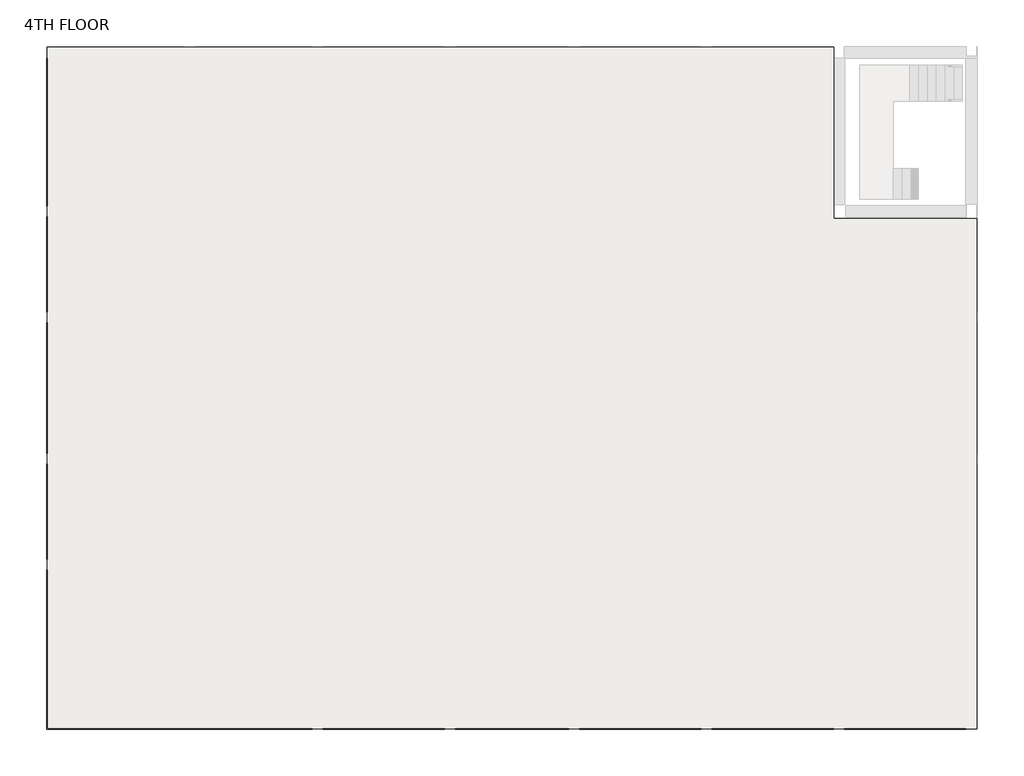
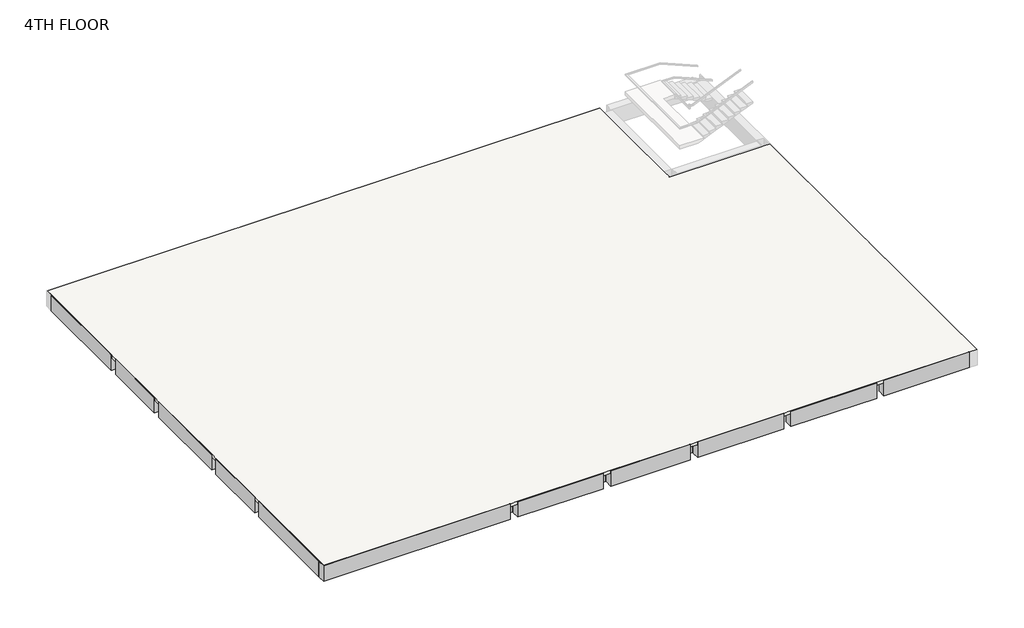
# One storey, part 1 of 2: 9 beams, 1 slab.
"""IFC4 building model written with IfcOpenShell, lengths in millimetres."""

from ifc_helpers import new_model, si_unit, frame, origin, place, context, project, spatial, polyline, outline, extrude, faceted_brep, element, save

model = new_model("IFC4")

# Units and contexts
model_context = context("Model", 3, world=origin())
ifc_project = project(units=[si_unit("LENGTHUNIT", "METRE", prefix="MILLI")], contexts=[model_context])

# Site, building, storey
site = spatial("IfcSite", under=ifc_project)
building = spatial("IfcBuilding", under=site)
storey = spatial("IfcBuildingStorey", under=building, Name="4TH FLOOR", Elevation=13716.0)

# Beams
placement = place(None, origin())
element("IfcBeam", 1, ObjectType="M_Concrete-Rectangular Beam : 400 x 800mm", at=placement, inside=storey, context=model_context, shape_type="Brep", body=[
    faceted_brep([(-25701.5491019, -6047.8309165, 13716.0), (-25701.5491019, -6447.8309165, 13716.0), (-16535.3491019, -6447.8309165, 13716.0), (-16535.3491019, -6425.6309165, 13716.0), (-25679.3491019, -6425.6309165, 13716.0), (-25679.3491019, -6047.8309165, 13716.0), (-25701.5491019, -6047.8309165, 12916.0), (-25679.3491019, -6047.8309165, 13563.6), (-25301.5491019, -6047.8309165, 13563.6), (-20977.1491019, -6047.8309165, 13563.6), (-20577.1491019, -6047.8309165, 13563.6), (-16557.5491019, -6047.8309165, 13563.6), (-16535.3491019, -6047.8309165, 13563.6), (-16535.3491019, -6047.8309165, 12916.0), (-16557.5491019, -6047.8309165, 12916.0), (-20577.1491019, -6047.8309165, 12916.0), (-20977.1491019, -6047.8309165, 12916.0), (-25301.5491019, -6047.8309165, 12916.0), (-25701.5491019, -6447.8309165, 12916.0), (-16535.3491019, -6447.8309165, 12916.0), (-25323.7491019, -6425.6309165, 12916.0), (-25323.7491019, -6070.0309165, 12916.0), (-25679.3491019, -6070.0309165, 12916.0), (-25679.3491019, -6425.6309165, 12916.0), (-20599.3491019, -6425.6309165, 12916.0), (-20599.3491019, -6070.0309165, 12916.0), (-20954.9491019, -6070.0309165, 12916.0), (-20954.9491019, -6425.6309165, 12916.0), (-25323.7491019, -6425.6309165, 13563.6), (-25323.7491019, -6070.0309165, 13563.6), (-16535.3491019, -6425.6309165, 13563.6), (-20599.3491019, -6425.6309165, 13563.6), (-20954.9491019, -6425.6309165, 13563.6), (-25679.3491019, -6425.6309165, 13563.6), (-25679.3491019, -6070.0309165, 13563.6), (-20599.3491019, -6070.0309165, 13563.6), (-20954.9491019, -6070.0309165, 13563.6)], [[[0, 1, 2, 3, 4, 5]], [[6, 0, 5, 7, 8, 9, 10, 11, 12, 13, 14, 15, 16, 17]], [[18, 6, 17, 16, 15, 14, 13, 19], [20, 21, 22, 23], [24, 25, 26, 27]], [[1, 18, 19, 2]], [[1, 0, 6, 18]], [[21, 20, 28, 29]], [[30, 31, 24, 27, 32, 28, 20, 23, 33, 4, 3]], [[4, 33, 23, 22, 34, 7, 5]], [[22, 21, 29, 34]], [[25, 24, 31, 35]], [[27, 26, 36, 32]], [[26, 25, 35, 36]], [[19, 13, 12, 30, 3, 2]], [[28, 32, 36, 35, 31, 30, 12, 11, 10, 9, 8, 7, 34, 29]]]),
    faceted_brep([(5997.6508981, -6447.8309165, 12916.0), (5997.6508981, -6047.8309165, 12916.0), (5997.6508981, -6047.8309165, 13563.6), (5997.6508981, -6425.6309165, 13563.6), (5997.6508981, -6425.6309165, 13716.0), (5997.6508981, -6447.8309165, 13716.0), (1803.4508981, -6047.8309165, 12916.0), (1803.4508981, -6447.8309165, 12916.0), (1803.4508981, -6447.8309165, 13716.0), (1803.4508981, -6425.6309165, 13716.0), (1803.4508981, -6425.6309165, 13563.6), (1803.4508981, -6047.8309165, 13563.6), (1825.6508981, -6047.8309165, 12916.0), (1825.6508981, -6047.8309165, 13563.6)], [[[0, 1, 2, 3, 4, 5]], [[6, 7, 8, 9, 10, 11]], [[8, 5, 4, 9]], [[1, 12, 6, 11, 13, 2]], [[1, 0, 7, 6, 12]], [[0, 5, 8, 7]], [[10, 3, 2, 13, 11]], [[3, 10, 9, 4]]]),
    faceted_brep([(-16179.7491019, -6047.8309165, 12916.0), (-16179.7491019, -6447.8309165, 12916.0), (-16179.7491019, -6447.8309165, 13716.0), (-16179.7491019, -6425.6309165, 13716.0), (-16179.7491019, -6425.6309165, 13563.6), (-16179.7491019, -6047.8309165, 13563.6), (-11963.3491019, -6447.8309165, 13716.0), (-11963.3491019, -6425.6309165, 13716.0), (-11963.3491019, -6047.8309165, 12916.0), (-11985.5491019, -6047.8309165, 12916.0), (-16157.5491019, -6047.8309165, 12916.0), (-16157.5491019, -6047.8309165, 13563.6), (-11985.5491019, -6047.8309165, 13563.6), (-11963.3491019, -6047.8309165, 13563.6), (-11963.3491019, -6447.8309165, 12916.0), (-11963.3491019, -6425.6309165, 13563.6)], [[[0, 1, 2, 3, 4, 5]], [[2, 6, 7, 3]], [[8, 9, 10, 0, 5, 11, 12, 13]], [[1, 0, 10, 9, 8, 14]], [[2, 1, 14, 6]], [[14, 8, 13, 15, 7, 6]], [[15, 4, 3, 7]], [[4, 15, 13, 12, 11, 5]]]),
    faceted_brep([(-11607.7491019, -6047.8309165, 12916.0), (-11607.7491019, -6447.8309165, 12916.0), (-11607.7491019, -6447.8309165, 13716.0), (-11607.7491019, -6425.6309165, 13716.0), (-11607.7491019, -6425.6309165, 13563.6), (-11607.7491019, -6047.8309165, 13563.6), (-7696.1491019, -6447.8309165, 13716.0), (-7696.1491019, -6425.6309165, 13716.0), (-7696.1491019, -6047.8309165, 12916.0), (-7718.3491019, -6047.8309165, 12916.0), (-11585.5491019, -6047.8309165, 12916.0), (-11585.5491019, -6047.8309165, 13563.6), (-7718.3491019, -6047.8309165, 13563.6), (-7696.1491019, -6047.8309165, 13563.6), (-7696.1491019, -6447.8309165, 12916.0), (-7696.1491019, -6425.6309165, 13563.6)], [[[0, 1, 2, 3, 4, 5]], [[2, 6, 7, 3]], [[8, 9, 10, 0, 5, 11, 12, 13]], [[1, 0, 10, 9, 8, 14]], [[2, 1, 14, 6]], [[14, 8, 13, 15, 7, 6]], [[15, 4, 3, 7]], [[4, 15, 13, 12, 11, 5]]]),
    faceted_brep([(-7340.5491019, -6047.8309165, 12916.0), (-7340.5491019, -6447.8309165, 12916.0), (-7340.5491019, -6447.8309165, 13716.0), (-7340.5491019, -6425.6309165, 13716.0), (-7340.5491019, -6425.6309165, 13563.6), (-7340.5491019, -6047.8309165, 13563.6), (-3124.1491019, -6447.8309165, 13716.0), (-3124.1491019, -6425.6309165, 13716.0), (-3124.1491019, -6047.8309165, 12916.0), (-3146.3491019, -6047.8309165, 12916.0), (-7318.3491019, -6047.8309165, 12916.0), (-7318.3491019, -6047.8309165, 13563.6), (-3146.3491019, -6047.8309165, 13563.6), (-3124.1491019, -6047.8309165, 13563.6), (-3124.1491019, -6447.8309165, 12916.0), (-3124.1491019, -6425.6309165, 13563.6)], [[[0, 1, 2, 3, 4, 5]], [[2, 6, 7, 3]], [[8, 9, 10, 0, 5, 11, 12, 13]], [[1, 0, 10, 9, 8, 14]], [[2, 1, 14, 6]], [[14, 8, 13, 15, 7, 6]], [[15, 4, 3, 7]], [[4, 15, 13, 12, 11, 5]]]),
    faceted_brep([(-2768.5491019, -6047.8309165, 12916.0), (-2768.5491019, -6447.8309165, 12916.0), (-2768.5491019, -6447.8309165, 13716.0), (-2768.5491019, -6425.6309165, 13716.0), (-2768.5491019, -6425.6309165, 13563.6), (-2768.5491019, -6047.8309165, 13563.6), (1447.8508981, -6447.8309165, 13716.0), (1447.8508981, -6425.6309165, 13716.0), (1447.8508981, -6047.8309165, 12916.0), (1425.6508981, -6047.8309165, 12916.0), (-2746.3491019, -6047.8309165, 12916.0), (-2746.3491019, -6047.8309165, 13563.6), (1425.6508981, -6047.8309165, 13563.6), (1447.8508981, -6047.8309165, 13563.6), (1447.8508981, -6447.8309165, 12916.0), (1447.8508981, -6425.6309165, 13563.6)], [[[0, 1, 2, 3, 4, 5]], [[2, 6, 7, 3]], [[8, 9, 10, 0, 5, 11, 12, 13]], [[1, 0, 10, 9, 8, 14]], [[2, 1, 14, 6]], [[14, 8, 13, 15, 7, 6]], [[15, 4, 3, 7]], [[4, 15, 13, 12, 11, 5]]]),
])
element("IfcBeam", 2, ObjectType="M_Concrete-Rectangular Beam : 400 x 800mm", at=placement, inside=storey, context=model_context, shape_type="Brep", body=[
    faceted_brep([(-25701.5491019, -939.2309165, 13716.0), (-25701.5491019, -6047.8309165, 13716.0), (-25679.3491019, -6047.8309165, 13716.0), (-25679.3491019, -939.2309165, 13716.0), (-25301.5491019, -6047.8309165, 12916.0), (-25301.5491019, -961.4309165, 12916.0), (-25301.5491019, -939.2309165, 12916.0), (-25301.5491019, -939.2309165, 13563.6), (-25301.5491019, -961.4309165, 13563.6), (-25301.5491019, -6047.8309165, 13563.6), (-25701.5491019, -6047.8309165, 12916.0), (-25701.5491019, -939.2309165, 12916.0), (-25679.3491019, -6047.8309165, 13563.6), (-25679.3491019, -939.2309165, 13563.6)], [[[0, 1, 2, 3]], [[4, 5, 6, 7, 8, 9]], [[4, 10, 11, 6, 5]], [[10, 1, 0, 11]], [[10, 4, 9, 12, 2, 1]], [[6, 11, 0, 3, 13, 7]], [[12, 13, 3, 2]], [[13, 12, 9, 8, 7]]]),
    faceted_brep([(-25301.5491019, 16716.9690835, 12916.0), (-25701.5491019, 16716.9690835, 12916.0), (-25701.5491019, 16716.9690835, 13716.0), (-25679.3491019, 16716.9690835, 13716.0), (-25679.3491019, 16716.9690835, 13563.6), (-25301.5491019, 16716.9690835, 13563.6), (-25701.5491019, 11608.3690835, 13716.0), (-25679.3491019, 11608.3690835, 13716.0), (-25301.5491019, 11608.3690835, 12916.0), (-25301.5491019, 11630.5690835, 12916.0), (-25301.5491019, 11630.5690835, 13563.6), (-25301.5491019, 11608.3690835, 13563.6), (-25701.5491019, 11608.3690835, 12916.0), (-25679.3491019, 11608.3690835, 13563.6)], [[[0, 1, 2, 3, 4, 5]], [[2, 6, 7, 3]], [[8, 9, 0, 5, 10, 11]], [[1, 0, 9, 8, 12]], [[2, 1, 12, 6]], [[12, 8, 11, 13, 7, 6]], [[4, 13, 11, 10, 5]], [[13, 4, 3, 7]]]),
    faceted_brep([(-25701.5491019, 7950.7690835, 12916.0), (-25301.5491019, 7950.7690835, 12916.0), (-25301.5491019, 7950.7690835, 13563.6), (-25679.3491019, 7950.7690835, 13563.6), (-25679.3491019, 7950.7690835, 13716.0), (-25701.5491019, 7950.7690835, 13716.0), (-25301.5491019, 11252.7690835, 12916.0), (-25701.5491019, 11252.7690835, 12916.0), (-25701.5491019, 11252.7690835, 13716.0), (-25679.3491019, 11252.7690835, 13716.0), (-25679.3491019, 11252.7690835, 13563.6), (-25301.5491019, 11252.7690835, 13563.6), (-25301.5491019, 7972.9690835, 13563.6), (-25301.5491019, 11230.5690835, 13563.6), (-25301.5491019, 7972.9690835, 12916.0), (-25301.5491019, 11230.5690835, 12916.0)], [[[0, 1, 2, 3, 4, 5]], [[6, 7, 8, 9, 10, 11]], [[10, 3, 2, 12, 13, 11]], [[3, 10, 9, 4]], [[8, 5, 4, 9]], [[1, 14, 15, 6, 11, 13, 12, 2]], [[1, 0, 7, 6, 15, 14]], [[0, 5, 8, 7]]]),
    faceted_brep([(-25301.5491019, 7595.1690835, 12916.0), (-25701.5491019, 7595.1690835, 12916.0), (-25701.5491019, 7595.1690835, 13716.0), (-25679.3491019, 7595.1690835, 13716.0), (-25679.3491019, 7595.1690835, 13563.6), (-25301.5491019, 7595.1690835, 13563.6), (-25701.5491019, 3073.9690835, 12916.0), (-25301.5491019, 3073.9690835, 12916.0), (-25301.5491019, 3073.9690835, 13563.6), (-25679.3491019, 3073.9690835, 13563.6), (-25679.3491019, 3073.9690835, 13716.0), (-25701.5491019, 3073.9690835, 13716.0), (-25301.5491019, 3096.1690835, 13563.6), (-25301.5491019, 7572.9690835, 13563.6), (-25301.5491019, 3096.1690835, 12916.0), (-25301.5491019, 7572.9690835, 12916.0)], [[[0, 1, 2, 3, 4, 5]], [[6, 7, 8, 9, 10, 11]], [[4, 9, 8, 12, 13, 5]], [[9, 4, 3, 10]], [[2, 11, 10, 3]], [[7, 14, 15, 0, 5, 13, 12, 8]], [[1, 0, 15, 14, 7, 6]], [[2, 1, 6, 11]]]),
    faceted_brep([(-25301.5491019, 2718.3690835, 12916.0), (-25701.5491019, 2718.3690835, 12916.0), (-25701.5491019, 2718.3690835, 13716.0), (-25679.3491019, 2718.3690835, 13716.0), (-25679.3491019, 2718.3690835, 13563.6), (-25301.5491019, 2718.3690835, 13563.6), (-25701.5491019, -583.6309165, 12916.0), (-25301.5491019, -583.6309165, 12916.0), (-25301.5491019, -583.6309165, 13563.6), (-25679.3491019, -583.6309165, 13563.6), (-25679.3491019, -583.6309165, 13716.0), (-25701.5491019, -583.6309165, 13716.0), (-25301.5491019, -561.4309165, 13563.6), (-25301.5491019, 2696.1690835, 13563.6), (-25301.5491019, -561.4309165, 12916.0), (-25301.5491019, 2696.1690835, 12916.0)], [[[0, 1, 2, 3, 4, 5]], [[6, 7, 8, 9, 10, 11]], [[4, 9, 8, 12, 13, 5]], [[9, 4, 3, 10]], [[2, 11, 10, 3]], [[7, 14, 15, 0, 5, 13, 12, 8]], [[0, 15, 14, 7, 6, 1]], [[11, 2, 1, 6]]]),
])
element("IfcBeam", 3, ObjectType="M_Concrete-Rectangular Beam : 400 x 800mm", at=placement, inside=storey, context=model_context, shape_type="SweptSolid", body=[
    extrude(outline(polyline([(-20577.1491019, -6047.8309165), (-20977.1491019, -6047.8309165), (-20977.1491019, -990.0309165), (-20577.1491019, -990.0309165), (-20577.1491019, -6047.8309165)])), frame((0.0, 0.0, 12916.0), z_axis=(0.0, 0.0, 1.0), x_axis=(1.0, 0.0, 0.0)), (0.0, 0.0, 1.0), 647.6),
    extrude(outline(polyline([(-20599.3491019, 16716.9690835), (-20577.1491019, 16716.9690835), (-20577.1491019, 11659.1690835), (-20977.1491019, 11659.1690835), (-20977.1491019, 16716.9690835), (-20954.9491019, 16716.9690835), (-20954.9491019, 16662.9690835), (-20599.3491019, 16662.9690835), (-20599.3491019, 16716.9690835)])), frame((0.0, 0.0, 12916.0), z_axis=(0.0, 0.0, 1.0), x_axis=(1.0, 0.0, 0.0)), (0.0, 0.0, 1.0), 647.6),
    extrude(outline(polyline([(-20977.1491019, 11201.9690835), (-20577.1491019, 11201.9690835), (-20577.1491019, 8001.5690835), (-20977.1491019, 8001.5690835), (-20977.1491019, 11201.9690835)])), frame((0.0, 0.0, 12916.0), z_axis=(0.0, 0.0, 1.0), x_axis=(1.0, 0.0, 0.0)), (0.0, 0.0, 1.0), 647.6),
    extrude(outline(polyline([(-20977.1491019, 7544.3690835), (-20577.1491019, 7544.3690835), (-20577.1491019, 3124.7690835), (-20977.1491019, 3124.7690835), (-20977.1491019, 7544.3690835)])), frame((0.0, 0.0, 12916.0), z_axis=(0.0, 0.0, 1.0), x_axis=(1.0, 0.0, 0.0)), (0.0, 0.0, 1.0), 647.6),
    extrude(outline(polyline([(-20977.1491019, 2667.5690835), (-20577.1491019, 2667.5690835), (-20577.1491019, -532.8309165), (-20977.1491019, -532.8309165), (-20977.1491019, 2667.5690835)])), frame((0.0, 0.0, 12916.0), z_axis=(0.0, 0.0, 1.0), x_axis=(1.0, 0.0, 0.0)), (0.0, 0.0, 1.0), 647.6),
])
element("IfcBeam", 4, ObjectType="M_Concrete-Rectangular Beam : 400 x 800mm", at=placement, inside=storey, context=model_context, shape_type="SweptSolid", body=[
    extrude(outline(polyline([(-16157.5491019, -6047.8309165), (-16179.7491019, -6047.8309165), (-16179.7491019, -6019.2309165), (-16535.3491019, -6019.2309165), (-16535.3491019, -6047.8309165), (-16557.5491019, -6047.8309165), (-16557.5491019, -990.0309165), (-16157.5491019, -990.0309165), (-16157.5491019, -6047.8309165)])), frame((0.0, 0.0, 12916.0), z_axis=(0.0, 0.0, 1.0), x_axis=(1.0, 0.0, 0.0)), (0.0, 0.0, 1.0), 647.6),
    extrude(outline(polyline([(-16179.7491019, 16716.9690835), (-16157.5491019, 16716.9690835), (-16157.5491019, 11659.1690835), (-16557.5491019, 11659.1690835), (-16557.5491019, 16716.9690835), (-16535.3491019, 16716.9690835), (-16535.3491019, 16688.3690835), (-16179.7491019, 16688.3690835), (-16179.7491019, 16716.9690835)])), frame((0.0, 0.0, 12916.0), z_axis=(0.0, 0.0, 1.0), x_axis=(1.0, 0.0, 0.0)), (0.0, 0.0, 1.0), 647.6),
    extrude(outline(polyline([(-16557.5491019, 11201.9690835), (-16157.5491019, 11201.9690835), (-16157.5491019, 8001.5690835), (-16557.5491019, 8001.5690835), (-16557.5491019, 11201.9690835)])), frame((0.0, 0.0, 12916.0), z_axis=(0.0, 0.0, 1.0), x_axis=(1.0, 0.0, 0.0)), (0.0, 0.0, 1.0), 647.6),
    extrude(outline(polyline([(-16557.5491019, 7544.3690835), (-16157.5491019, 7544.3690835), (-16157.5491019, 3124.7690835), (-16557.5491019, 3124.7690835), (-16557.5491019, 7544.3690835)])), frame((0.0, 0.0, 12916.0), z_axis=(0.0, 0.0, 1.0), x_axis=(1.0, 0.0, 0.0)), (0.0, 0.0, 1.0), 647.6),
    extrude(outline(polyline([(-16557.5491019, 2667.5690835), (-16157.5491019, 2667.5690835), (-16157.5491019, -532.8309165), (-16557.5491019, -532.8309165), (-16557.5491019, 2667.5690835)])), frame((0.0, 0.0, 12916.0), z_axis=(0.0, 0.0, 1.0), x_axis=(1.0, 0.0, 0.0)), (0.0, 0.0, 1.0), 647.6),
])
element("IfcBeam", 5, ObjectType="M_Concrete-Rectangular Beam : 400 x 800mm", at=placement, inside=storey, context=model_context, shape_type="SweptSolid", body=[
    extrude(outline(polyline([(-11585.5491019, -6047.8309165), (-11607.7491019, -6047.8309165), (-11607.7491019, -6019.2309165), (-11963.3491019, -6019.2309165), (-11963.3491019, -6047.8309165), (-11985.5491019, -6047.8309165), (-11985.5491019, -990.0309165), (-11585.5491019, -990.0309165), (-11585.5491019, -6047.8309165)])), frame((0.0, 0.0, 12916.0), z_axis=(0.0, 0.0, 1.0), x_axis=(1.0, 0.0, 0.0)), (0.0, 0.0, 1.0), 647.6),
    extrude(outline(polyline([(-11607.7491019, 16716.9690835), (-11585.5491019, 16716.9690835), (-11585.5491019, 11659.1690835), (-11985.5491019, 11659.1690835), (-11985.5491019, 16716.9690835), (-11963.3491019, 16716.9690835), (-11963.3491019, 16688.3690835), (-11607.7491019, 16688.3690835), (-11607.7491019, 16716.9690835)])), frame((0.0, 0.0, 12916.0), z_axis=(0.0, 0.0, 1.0), x_axis=(1.0, 0.0, 0.0)), (0.0, 0.0, 1.0), 647.6),
    extrude(outline(polyline([(-11985.5491019, 11201.9690835), (-11585.5491019, 11201.9690835), (-11585.5491019, 8001.5690835), (-11985.5491019, 8001.5690835), (-11985.5491019, 11201.9690835)])), frame((0.0, 0.0, 12916.0), z_axis=(0.0, 0.0, 1.0), x_axis=(1.0, 0.0, 0.0)), (0.0, 0.0, 1.0), 647.6),
    extrude(outline(polyline([(-11985.5491019, 7544.3690835), (-11585.5491019, 7544.3690835), (-11585.5491019, 3124.7690835), (-11985.5491019, 3124.7690835), (-11985.5491019, 7544.3690835)])), frame((0.0, 0.0, 12916.0), z_axis=(0.0, 0.0, 1.0), x_axis=(1.0, 0.0, 0.0)), (0.0, 0.0, 1.0), 647.6),
    extrude(outline(polyline([(-11585.5491019, -532.8309165), (-11985.5491019, -532.8309165), (-11985.5491019, 2667.5690835), (-11585.5491019, 2667.5690835), (-11585.5491019, -532.8309165)])), frame((0.0, 0.0, 12916.0), z_axis=(0.0, 0.0, 1.0), x_axis=(1.0, 0.0, 0.0)), (0.0, 0.0, 1.0), 647.6),
])
element("IfcBeam", 6, ObjectType="M_Concrete-Rectangular Beam : 400 x 800mm", at=placement, inside=storey, context=model_context, shape_type="SweptSolid", body=[
    extrude(outline(polyline([(-7318.3491019, -6047.8309165), (-7340.5491019, -6047.8309165), (-7340.5491019, -6019.2309165), (-7696.1491019, -6019.2309165), (-7696.1491019, -6047.8309165), (-7718.3491019, -6047.8309165), (-7718.3491019, -990.0309165), (-7318.3491019, -990.0309165), (-7318.3491019, -6047.8309165)])), frame((0.0, 0.0, 12916.0), z_axis=(0.0, 0.0, 1.0), x_axis=(1.0, 0.0, 0.0)), (0.0, 0.0, 1.0), 647.6),
    extrude(outline(polyline([(-7340.5491019, 16716.9690835), (-7318.3491019, 16716.9690835), (-7318.3491019, 11659.1690835), (-7718.3491019, 11659.1690835), (-7718.3491019, 16716.9690835), (-7696.1491019, 16716.9690835), (-7696.1491019, 16688.3690835), (-7340.5491019, 16688.3690835), (-7340.5491019, 16716.9690835)])), frame((0.0, 0.0, 12916.0), z_axis=(0.0, 0.0, 1.0), x_axis=(1.0, 0.0, 0.0)), (0.0, 0.0, 1.0), 647.6),
    extrude(outline(polyline([(-7718.3491019, 7544.3690835), (-7318.3491019, 7544.3690835), (-7318.3491019, 3124.7690835), (-7718.3491019, 3124.7690835), (-7718.3491019, 7544.3690835)])), frame((0.0, 0.0, 12916.0), z_axis=(0.0, 0.0, 1.0), x_axis=(1.0, 0.0, 0.0)), (0.0, 0.0, 1.0), 647.6),
    extrude(outline(polyline([(-7318.3491019, 8001.5690835), (-7718.3491019, 8001.5690835), (-7718.3491019, 11201.9690835), (-7318.3491019, 11201.9690835), (-7318.3491019, 8001.5690835)])), frame((0.0, 0.0, 12916.0), z_axis=(0.0, 0.0, 1.0), x_axis=(1.0, 0.0, 0.0)), (0.0, 0.0, 1.0), 647.6),
    extrude(outline(polyline([(-7318.3491019, -532.8309165), (-7718.3491019, -532.8309165), (-7718.3491019, 2667.5690835), (-7318.3491019, 2667.5690835), (-7318.3491019, -532.8309165)])), frame((0.0, 0.0, 12916.0), z_axis=(0.0, 0.0, 1.0), x_axis=(1.0, 0.0, 0.0)), (0.0, 0.0, 1.0), 647.6),
])
element("IfcBeam", 7, ObjectType="M_Concrete-Rectangular Beam : 400 x 800mm", at=placement, inside=storey, context=model_context, shape_type="SweptSolid", body=[
    extrude(outline(polyline([(-25301.5491019, 3073.9690835), (-25301.5491019, 3096.1690835), (-21005.7491019, 3096.1690835), (-21005.7491019, 2696.1690835), (-25301.5491019, 2696.1690835), (-25301.5491019, 2718.3690835), (-25272.9491019, 2718.3690835), (-25272.9491019, 3073.9690835), (-25301.5491019, 3073.9690835)])), frame((0.0, 0.0, 12916.0), z_axis=(0.0, 0.0, 1.0), x_axis=(1.0, 0.0, 0.0)), (0.0, 0.0, 1.0), 647.6),
    extrude(outline(polyline([(5997.6508981, 3096.1690835), (5997.6508981, 3073.9690835), (5969.0508981, 3073.9690835), (5969.0508981, 2718.3690835), (5997.6508981, 2718.3690835), (5997.6508981, 2696.1690835), (1854.2508981, 2696.1690835), (1854.2508981, 3096.1690835), (5997.6508981, 3096.1690835)])), frame((0.0, 0.0, 12916.0), z_axis=(0.0, 0.0, 1.0), x_axis=(1.0, 0.0, 0.0)), (0.0, 0.0, 1.0), 647.6),
    extrude(outline(polyline([(-20548.5491019, 2696.1690835), (-20548.5491019, 3096.1690835), (-16586.1491019, 3096.1690835), (-16586.1491019, 2696.1690835), (-20548.5491019, 2696.1690835)])), frame((0.0, 0.0, 12916.0), z_axis=(0.0, 0.0, 1.0), x_axis=(1.0, 0.0, 0.0)), (0.0, 0.0, 1.0), 647.6),
    extrude(outline(polyline([(-16128.9491019, 2696.1690835), (-16128.9491019, 3096.1690835), (-12014.1491019, 3096.1690835), (-12014.1491019, 2696.1690835), (-16128.9491019, 2696.1690835)])), frame((0.0, 0.0, 12916.0), z_axis=(0.0, 0.0, 1.0), x_axis=(1.0, 0.0, 0.0)), (0.0, 0.0, 1.0), 647.6),
    extrude(outline(polyline([(1397.0508981, 3096.1690835), (1397.0508981, 2696.1690835), (-2717.7491019, 2696.1690835), (-2717.7491019, 3096.1690835), (1397.0508981, 3096.1690835)])), frame((0.0, 0.0, 12916.0), z_axis=(0.0, 0.0, 1.0), x_axis=(1.0, 0.0, 0.0)), (0.0, 0.0, 1.0), 647.6),
    extrude(outline(polyline([(-3174.9491019, 3096.1690835), (-3174.9491019, 2696.1690835), (-7289.7491019, 2696.1690835), (-7289.7491019, 3096.1690835), (-3174.9491019, 3096.1690835)])), frame((0.0, 0.0, 12916.0), z_axis=(0.0, 0.0, 1.0), x_axis=(1.0, 0.0, 0.0)), (0.0, 0.0, 1.0), 647.6),
    extrude(outline(polyline([(-7746.9491019, 3096.1690835), (-7746.9491019, 2696.1690835), (-11556.9491019, 2696.1690835), (-11556.9491019, 3096.1690835), (-7746.9491019, 3096.1690835)])), frame((0.0, 0.0, 12916.0), z_axis=(0.0, 0.0, 1.0), x_axis=(1.0, 0.0, 0.0)), (0.0, 0.0, 1.0), 647.6),
])
element("IfcBeam", 8, ObjectType="M_Concrete-Rectangular Beam : 400 x 800mm", at=placement, inside=storey, context=model_context, shape_type="SweptSolid", body=[
    extrude(outline(polyline([(-25301.5491019, -583.6309165), (-25301.5491019, -561.4309165), (-21005.7491019, -561.4309165), (-21005.7491019, -961.4309165), (-25301.5491019, -961.4309165), (-25301.5491019, -939.2309165), (-25247.5491019, -939.2309165), (-25247.5491019, -583.6309165), (-25301.5491019, -583.6309165)])), frame((0.0, 0.0, 12916.0), z_axis=(0.0, 0.0, 1.0), x_axis=(1.0, 0.0, 0.0)), (0.0, 0.0, 1.0), 647.6),
    extrude(outline(polyline([(5997.6508981, -561.4309165), (5997.6508981, -961.4309165), (1854.2508981, -961.4309165), (1854.2508981, -561.4309165), (5997.6508981, -561.4309165)])), frame((0.0, 0.0, 12916.0), z_axis=(0.0, 0.0, 1.0), x_axis=(1.0, 0.0, 0.0)), (0.0, 0.0, 1.0), 647.6),
    extrude(outline(polyline([(-20548.5491019, -961.4309165), (-20548.5491019, -561.4309165), (-16586.1491019, -561.4309165), (-16586.1491019, -961.4309165), (-20548.5491019, -961.4309165)])), frame((0.0, 0.0, 12916.0), z_axis=(0.0, 0.0, 1.0), x_axis=(1.0, 0.0, 0.0)), (0.0, 0.0, 1.0), 647.6),
    extrude(outline(polyline([(-16128.9491019, -961.4309165), (-16128.9491019, -561.4309165), (-12014.1491019, -561.4309165), (-12014.1491019, -961.4309165), (-16128.9491019, -961.4309165)])), frame((0.0, 0.0, 12916.0), z_axis=(0.0, 0.0, 1.0), x_axis=(1.0, 0.0, 0.0)), (0.0, 0.0, 1.0), 647.6),
    extrude(outline(polyline([(-11556.9491019, -961.4309165), (-11556.9491019, -561.4309165), (-7746.9491019, -561.4309165), (-7746.9491019, -961.4309165), (-11556.9491019, -961.4309165)])), frame((0.0, 0.0, 12916.0), z_axis=(0.0, 0.0, 1.0), x_axis=(1.0, 0.0, 0.0)), (0.0, 0.0, 1.0), 647.6),
    extrude(outline(polyline([(-7289.7491019, -961.4309165), (-7289.7491019, -561.4309165), (-3174.9491019, -561.4309165), (-3174.9491019, -961.4309165), (-7289.7491019, -961.4309165)])), frame((0.0, 0.0, 12916.0), z_axis=(0.0, 0.0, 1.0), x_axis=(1.0, 0.0, 0.0)), (0.0, 0.0, 1.0), 647.6),
    extrude(outline(polyline([(-2717.7491019, -961.4309165), (-2717.7491019, -561.4309165), (1397.0508981, -561.4309165), (1397.0508981, -961.4309165), (-2717.7491019, -961.4309165)])), frame((0.0, 0.0, 12916.0), z_axis=(0.0, 0.0, 1.0), x_axis=(1.0, 0.0, 0.0)), (0.0, 0.0, 1.0), 647.6),
])
element("IfcBeam", 9, ObjectType="M_Concrete-Rectangular Beam : 400 x 800mm", at=placement, inside=storey, context=model_context, shape_type="SweptSolid", body=[
    extrude(outline(polyline([(-25301.5491019, 7950.7690835), (-25301.5491019, 7972.9690835), (-21005.7491019, 7972.9690835), (-21005.7491019, 7572.9690835), (-25301.5491019, 7572.9690835), (-25301.5491019, 7595.1690835), (-25272.9491019, 7595.1690835), (-25272.9491019, 7950.7690835), (-25301.5491019, 7950.7690835)])), frame((0.0, 0.0, 12916.0), z_axis=(0.0, 0.0, 1.0), x_axis=(1.0, 0.0, 0.0)), (0.0, 0.0, 1.0), 647.6),
    extrude(outline(polyline([(5997.6508981, 7972.9690835), (5997.6508981, 7950.7690835), (5969.0508981, 7950.7690835), (5969.0508981, 7595.1690835), (5997.6508981, 7595.1690835), (5997.6508981, 7572.9690835), (1854.2508981, 7572.9690835), (1854.2508981, 7972.9690835), (5997.6508981, 7972.9690835)])), frame((0.0, 0.0, 12916.0), z_axis=(0.0, 0.0, 1.0), x_axis=(1.0, 0.0, 0.0)), (0.0, 0.0, 1.0), 647.6),
    extrude(outline(polyline([(-7289.7491019, 7572.9690835), (-7289.7491019, 7972.9690835), (-3174.9491019, 7972.9690835), (-3174.9491019, 7572.9690835), (-7289.7491019, 7572.9690835)])), frame((0.0, 0.0, 12916.0), z_axis=(0.0, 0.0, 1.0), x_axis=(1.0, 0.0, 0.0)), (0.0, 0.0, 1.0), 647.6),
    extrude(outline(polyline([(-7746.9491019, 7972.9690835), (-7746.9491019, 7572.9690835), (-11556.9491019, 7572.9690835), (-11556.9491019, 7972.9690835), (-7746.9491019, 7972.9690835)])), frame((0.0, 0.0, 12916.0), z_axis=(0.0, 0.0, 1.0), x_axis=(1.0, 0.0, 0.0)), (0.0, 0.0, 1.0), 647.6),
    extrude(outline(polyline([(1397.0508981, 7972.9690835), (1397.0508981, 7572.9690835), (-2717.7491019, 7572.9690835), (-2717.7491019, 7972.9690835), (1397.0508981, 7972.9690835)])), frame((0.0, 0.0, 12916.0), z_axis=(0.0, 0.0, 1.0), x_axis=(1.0, 0.0, 0.0)), (0.0, 0.0, 1.0), 647.6),
    extrude(outline(polyline([(-12014.1491019, 7972.9690835), (-12014.1491019, 7572.9690835), (-16128.9491019, 7572.9690835), (-16128.9491019, 7972.9690835), (-12014.1491019, 7972.9690835)])), frame((0.0, 0.0, 12916.0), z_axis=(0.0, 0.0, 1.0), x_axis=(1.0, 0.0, 0.0)), (0.0, 0.0, 1.0), 647.6),
    extrude(outline(polyline([(-16586.1491019, 7972.9690835), (-16586.1491019, 7572.9690835), (-20548.5491019, 7572.9690835), (-20548.5491019, 7972.9690835), (-16586.1491019, 7972.9690835)])), frame((0.0, 0.0, 12916.0), z_axis=(0.0, 0.0, 1.0), x_axis=(1.0, 0.0, 0.0)), (0.0, 0.0, 1.0), 647.6),
])

# Slab
element("IfcSlab", 10, ObjectType="6\" Foundation Slab", at=placement, inside=storey, context=model_context, shape_type="Brep", body=[
    faceted_brep([(6375.4508981, -6425.6309165, 13563.6), (6019.8508981, -6425.6309165, 13563.6), (5997.6508981, -6425.6309165, 13563.6), (1803.4508981, -6425.6309165, 13563.6), (1447.8508981, -6425.6309165, 13563.6), (-2768.5491019, -6425.6309165, 13563.6), (-3124.1491019, -6425.6309165, 13563.6), (-7340.5491019, -6425.6309165, 13563.6), (-7696.1491019, -6425.6309165, 13563.6), (-11607.7491019, -6425.6309165, 13563.6), (-11963.3491019, -6425.6309165, 13563.6), (-16179.7491019, -6425.6309165, 13563.6), (-16535.3491019, -6425.6309165, 13563.6), (-20599.3491019, -6425.6309165, 13563.6), (-20954.9491019, -6425.6309165, 13563.6), (-25323.7491019, -6425.6309165, 13563.6), (-25679.3491019, -6425.6309165, 13563.6), (-25679.3491019, -6070.0309165, 13563.6), (-25679.3491019, -6047.8309165, 13563.6), (-25679.3491019, -939.2309165, 13563.6), (-25679.3491019, -583.6309165, 13563.6), (-25679.3491019, 2718.3690835, 13563.6), (-25679.3491019, 3073.9690835, 13563.6), (-25679.3491019, 7595.1690835, 13563.6), (-25679.3491019, 7950.7690835, 13563.6), (-25679.3491019, 11252.7690835, 13563.6), (-25679.3491019, 11608.3690835, 13563.6), (-25679.3491019, 16716.9690835, 13563.6), (-25679.3491019, 16739.1690835, 13563.6), (-25679.3491019, 17094.7690835, 13563.6), (-25323.7491019, 17094.7690835, 13563.6), (-20954.9491019, 17094.7690835, 13563.6), (-20599.3491019, 17094.7690835, 13563.6), (-16535.3491019, 17094.7690835, 13563.6), (-16179.7491019, 17094.7690835, 13563.6), (-11963.3491019, 17094.7690835, 13563.6), (-11607.7491019, 17094.7690835, 13563.6), (-7696.1491019, 17094.7690835, 13563.6), (-7340.5491019, 17094.7690835, 13563.6), (-3124.1491019, 17094.7690835, 13563.6), (-2768.5491019, 17094.7690835, 13563.6), (1447.8508981, 17094.7690835, 13563.6), (1447.8508981, 16716.9690835, 13563.6), (1447.8508981, 16713.7690835, 13563.6), (1447.8508981, 11659.1690835, 13563.6), (1447.8508981, 11201.9690835, 13563.6), (1447.8508981, 11176.5690835, 13563.6), (1825.6508981, 11176.5690835, 13563.6), (5997.6508981, 11176.5690835, 13563.6), (6019.8508981, 11176.5690835, 13563.6), (6375.4508981, 11176.5690835, 13563.6), (6375.4508981, 7950.7690835, 13563.6), (6375.4508981, 7595.1690835, 13563.6), (6375.4508981, 3073.9690835, 13563.6), (6375.4508981, 2718.3690835, 13563.6), (6375.4508981, -507.4309165, 13563.6), (6375.4508981, -1015.4309165, 13563.6), (6375.4508981, -6070.0309165, 13563.6), (-25679.3491019, -6425.6309165, 13716.0), (-16535.3491019, -6425.6309165, 13716.0), (-16179.7491019, -6425.6309165, 13716.0), (-11963.3491019, -6425.6309165, 13716.0), (-11607.7491019, -6425.6309165, 13716.0), (-7696.1491019, -6425.6309165, 13716.0), (-7340.5491019, -6425.6309165, 13716.0), (-3124.1491019, -6425.6309165, 13716.0), (-2768.5491019, -6425.6309165, 13716.0), (1447.8508981, -6425.6309165, 13716.0), (1803.4508981, -6425.6309165, 13716.0), (5997.6508981, -6425.6309165, 13716.0), (6375.4508981, -6425.6309165, 13716.0), (6375.4508981, 2718.3690835, 13716.0), (6375.4508981, 3073.9690835, 13716.0), (6375.4508981, 7595.1690835, 13716.0), (6375.4508981, 7950.7690835, 13716.0), (6375.4508981, 11176.5690835, 13716.0), (6019.8508981, 11176.5690835, 13716.0), (5997.6508981, 11176.5690835, 13716.0), (1825.6508981, 11176.5690835, 13716.0), (1447.8508981, 11176.5690835, 13716.0), (1447.8508981, 11201.9690835, 13716.0), (1447.8508981, 11659.1690835, 13716.0), (1447.8508981, 16713.7690835, 13716.0), (1447.8508981, 17094.7690835, 13716.0), (-2768.5491019, 17094.7690835, 13716.0), (-3124.1491019, 17094.7690835, 13716.0), (-7340.5491019, 17094.7690835, 13716.0), (-7696.1491019, 17094.7690835, 13716.0), (-11607.7491019, 17094.7690835, 13716.0), (-11963.3491019, 17094.7690835, 13716.0), (-16179.7491019, 17094.7690835, 13716.0), (-16535.3491019, 17094.7690835, 13716.0), (-20599.3491019, 17094.7690835, 13716.0), (-20954.9491019, 17094.7690835, 13716.0), (-25679.3491019, 17094.7690835, 13716.0), (-25679.3491019, 16716.9690835, 13716.0), (-25679.3491019, 11608.3690835, 13716.0), (-25679.3491019, 11252.7690835, 13716.0), (-25679.3491019, 7950.7690835, 13716.0), (-25679.3491019, 7595.1690835, 13716.0), (-25679.3491019, 3073.9690835, 13716.0), (-25679.3491019, 2718.3690835, 13716.0), (-25679.3491019, -583.6309165, 13716.0), (-25679.3491019, -939.2309165, 13716.0), (-25679.3491019, -6047.8309165, 13716.0)], [[[0, 1, 2, 3, 4, 5, 6, 7, 8, 9, 10, 11, 12, 13, 14, 15, 16, 17, 18, 19, 20, 21, 22, 23, 24, 25, 26, 27, 28, 29, 30, 31, 32, 33, 34, 35, 36, 37, 38, 39, 40, 41, 42, 43, 44, 45, 46, 47, 48, 49, 50, 51, 52, 53, 54, 55, 56, 57]], [[58, 59, 60, 61, 62, 63, 64, 65, 66, 67, 68, 69, 70, 71, 72, 73, 74, 75, 76, 77, 78, 79, 80, 81, 82, 83, 84, 85, 86, 87, 88, 89, 90, 91, 92, 93, 94, 95, 96, 97, 98, 99, 100, 101, 102, 103, 104]], [[70, 0, 57, 56, 55, 54, 53, 52, 51, 50, 75, 74, 73, 72, 71]], [[16, 15, 14, 13, 12, 11, 10, 9, 8, 7, 6, 5, 4, 3, 2, 1, 0, 70, 69, 68, 67, 66, 65, 64, 63, 62, 61, 60, 59, 58]], [[29, 28, 27, 26, 25, 24, 23, 22, 21, 20, 19, 18, 17, 16, 58, 104, 103, 102, 101, 100, 99, 98, 97, 96, 95, 94]], [[29, 94, 93, 92, 91, 90, 89, 88, 87, 86, 85, 84, 83, 41, 40, 39, 38, 37, 36, 35, 34, 33, 32, 31, 30]], [[79, 46, 45, 44, 43, 42, 41, 83, 82, 81, 80]], [[46, 79, 78, 77, 76, 75, 50, 49, 48, 47]]]),
])

save(model, "model.ifc")

# Revit data of these elements
# Type "M_Concrete-Rectangular Beam : 400 x 800mm"
#   Length [instance default] = 5' - 0"
#   b = 1' - 3.74803"
#   h = 2' - 7.49606"
#   Structural Material [instance default] = Concrete, Cast-in-Place gray
#   Assembly Code = ""
# Type "6\" Foundation Slab"
#   Layers, outside or top first: 0' - 6" "Concrete, Cast-in-Place gray" (function 1)
# Elements 1, 2 (IfcBeam, "M_Concrete-Rectangular Beam : 400 x 800mm")
#   Structural Material = Concrete, Cast-in-Place gray
#   Phase Created = New Construction
#   Materials on its faces: "Concrete, Cast-in-Place gray"
# Elements 3, 4, 5, 6, 7, 8, 9 (IfcBeam, "M_Concrete-Rectangular Beam : 400 x 800mm")
#   Comments = ""
#   Structural Material = Concrete, Cast-in-Place gray
#   Phase Created = New Construction
#   Materials on its faces: "Concrete, Cast-in-Place gray"
# Element 10 (IfcSlab, "6\" Foundation Slab")
#   Height Offset From Level = 0' - 0"
#   built-in parameter 1001954 = 1
#   Phase Created = New Construction
#   Materials on its faces: "Concrete, Cast-in-Place gray"
# Materials
#   "Concrete, Cast-in-Place gray": class "Concrete", colour RGB 192 192 192, transparency 0, Description = "Cast-in-place concrete", Cost = 0
